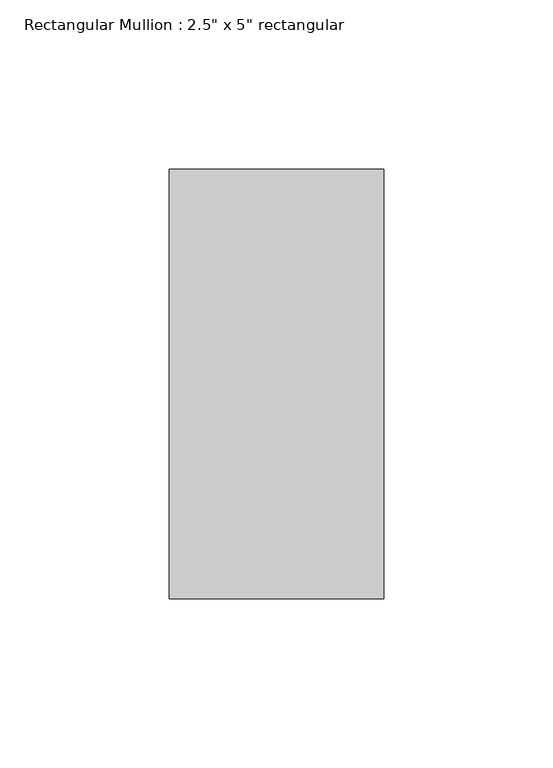
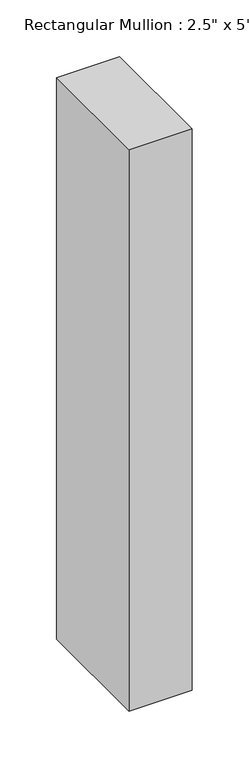
"""IFC4 building model written with IfcOpenShell, lengths in millimetres: member geometry."""

from ifc_helpers import new_model, si_unit, frame, origin, place, context, project, spatial, polyline, outline, extrude, source, transform, mapped, element, save


def member_94122dd8(model_context):
    return source(origin(), model_context, "Body", "SweptSolid", [
        extrude(outline(polyline([(0.0, 63.5), (0.0, -63.5), (-63.5, -63.5), (-63.5, 63.5), (0.0, 63.5)])), frame((0.0, 0.0, -601.1333333), z_axis=(0.0, 0.0, 1.0), x_axis=(1.0, 0.0, 0.0)), (0.0, 0.0, 1.0), 601.1333333),
    ])


if __name__ == "__main__":
    model = new_model("IFC4")
    model_context = context("Model", 3, world=origin())
    ifc_project = project(units=[si_unit("LENGTHUNIT", "METRE", prefix="MILLI")], contexts=[model_context])
    site = spatial("IfcSite", under=ifc_project)
    building = spatial("IfcBuilding", under=site)
    placement = place(None, origin())
    member_shape = member_94122dd8(model_context)
    element("IfcMember", 1, ObjectType="Rectangular Mullion : 2.5\" x 5\" rectangular", at=placement, inside=building, context=model_context, shape_type="MappedRepresentation", body=[
        mapped(member_shape, transform((0.0, 0.0, 0.0), x_axis=(1.0, 0.0, 0.0), y_axis=(0.0, 1.0, 0.0), z_axis=(0.0, 0.0, 1.0))),
    ])
    save(model, "model.ifc")

# Revit data of these elements
# Type "Rectangular Mullion : 2.5\" x 5\" rectangular"
#   built-in parameter 1007304 = 0.416667 (stored number, unit not read)
#   built-in parameter 1007301 = 0.104167 (stored number, unit not read)
#   built-in parameter 1007300 = 0.104167 (stored number, unit not read)
# Element 1 (IfcMember, "Rectangular Mullion : 2.5\" x 5\" rectangular")
#   Materials on its faces: "Aluminum"
# Materials
#   "Aluminum": class "Metal", colour RGB 247 247 247, transparency 0, Description = "Aluminum 6061", Cost = 0
